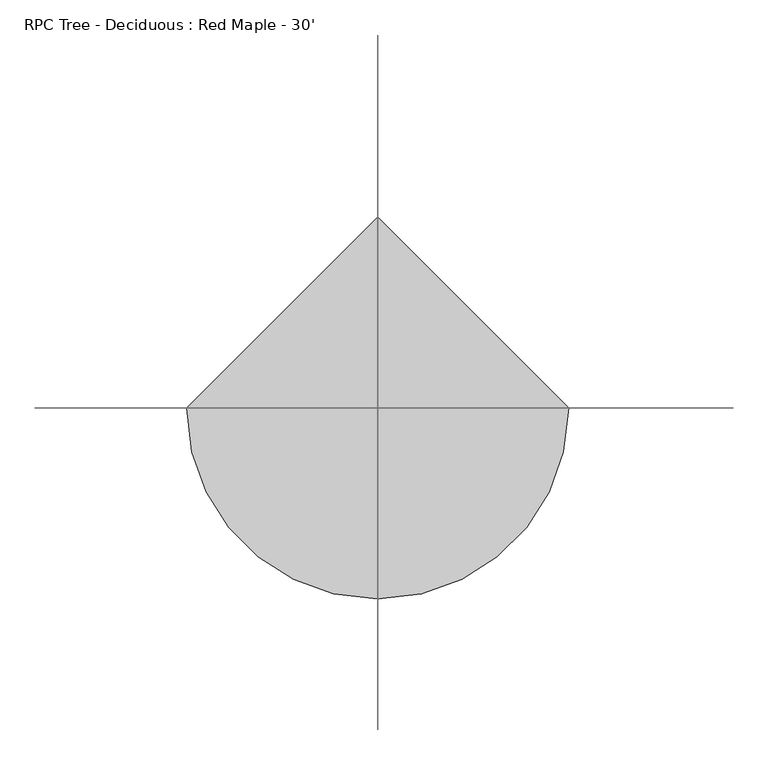
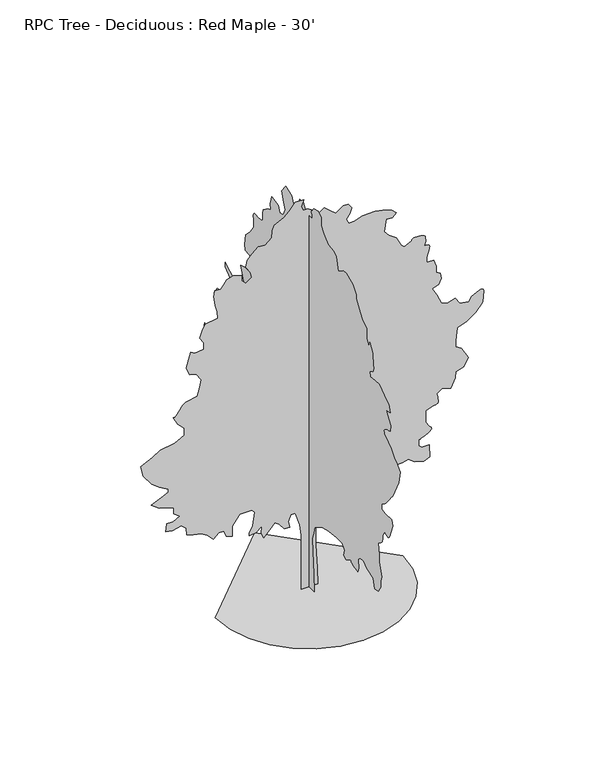
"""IFC4 building model written with IfcOpenShell, lengths in millimetres: geographic element geometry, RPC Tree - Deciduous : Red Maple - 30'."""

from ifc_helpers import new_model, si_unit, origin, place, context, project, spatial, triangles, source, transform, mapped, element, save


def rpc_tree_deciduous_red_maple_30_cba750cc(model_context):
    return source(origin(), model_context, "Body", "Tessellation", [
        triangles([(5.9e-06, 200.5240248, 0.0131599), (5.9e-06, -200.5423013, 0.0131599), (5.9e-06, -173.8047255, 401.079007), (5.9e-06, -147.0663684, 922.4677488), (5.9e-06, -133.6980892, 1216.5822092), (5.9e-06, -173.8047255, 1363.6407475), (5.9e-06, -227.2806583, 1537.4352264), (5.9e-06, -320.8632274, 1590.9124855), (5.9e-06, -534.7644153, 1711.2323215), (5.9e-06, -762.0361897, 1764.7071098), (5.9e-06, -1069.5212002, 1804.8136734), (5.9e-06, -1283.4223881, 1804.8136734), (5.9e-06, -1377.0037399, 1697.8617714), (5.9e-06, -1336.897031, 1550.8033058), (5.9e-06, -1443.848933, 1510.6967422), (5.9e-06, -1617.6460281, 1604.2805649), (5.9e-06, -1620.762553, 1592.8200726), (5.9e-06, -1625.400642, 1581.362051), (5.9e-06, -1633.0790977, 1569.9041748), (5.9e-06, -1645.319339, 1558.4436825), (5.9e-06, -1663.6378429, 1546.9856609), (5.9e-06, -1689.5560284, 1535.5251686), (5.9e-06, -1724.595314, 1524.0672924), (5.9e-06, -1761.1942429, 1514.1662979), (5.9e-06, -1791.4812023, 1507.0721088), (5.9e-06, -1816.5027855, 1502.3197826), (5.9e-06, -1837.3156139, 1499.4343483), (5.9e-06, -1854.971077, 1497.9534794), (5.9e-06, -1870.5234707, 1497.4074371), (5.9e-06, -1885.021859, 1497.3286629), (5.9e-06, -1911.7604885, 1590.9124855), (5.9e-06, -1898.3924091, 1791.445594), (5.9e-06, -1978.6056816, 1871.6588665), (5.9e-06, -2112.293597, 1885.0269459), (5.9e-06, -2219.245499, 1778.0750439), (5.9e-06, -2473.2533958, 1697.8617714), (5.9e-06, -2540.1036758, 1497.3286629), (5.9e-06, -2660.4236572, 1510.6967422), (5.9e-06, -2767.3575371, 1671.125758), (5.9e-06, -2767.3575371, 1804.8136734), (5.9e-06, -2794.1038696, 1911.7655754), (5.9e-06, -2700.5302208, 2219.2479698), (5.9e-06, -2700.5302208, 2393.0450649), (5.9e-06, -2673.7838882, 2660.4236572), (5.9e-06, -2676.8572472, 2660.5759735), (5.9e-06, -2681.2261665, 2661.668058), (5.9e-06, -2688.1603363, 2664.6399696), (5.9e-06, -2698.9553169, 2670.4056061), (5.9e-06, -2714.9066689, 2679.9053169), (5.9e-06, -2737.284082, 2694.1038689), (5.9e-06, -2767.3575371, 2713.8904518), (5.9e-06, -2796.66912, 2738.3761665), (5.9e-06, -2816.8623642, 2765.6558968), (5.9e-06, -2829.4607231, 2795.2721123), (5.9e-06, -2835.9629425, 2826.7681549), (5.9e-06, -2837.9189278, 2859.6612053), (5.9e-06, -2836.8265526, 2893.4940239), (5.9e-06, -2834.2104332, 2927.8096619), (5.9e-06, -2914.423851, 3061.4898743), (5.9e-06, -2945.8434448, 3041.8556076), (5.9e-06, -2976.6790627, 3024.6598549), (5.9e-06, -3006.3211487, 3012.3917084), (5.9e-06, -3034.2357239, 3007.4641022), (5.9e-06, -3059.8135231, 3012.3917084), (5.9e-06, -3082.4449905, 3029.5618813), (5.9e-06, -3101.5964378, 3061.4898743), (5.9e-06, -3235.2766502, 3382.3429642), (5.9e-06, -3195.1700867, 3516.0231766), (5.9e-06, -2941.1698929, 3502.6629456), (5.9e-06, -2794.1038696, 3516.0231766), (5.9e-06, -2807.4641006, 3649.7289688), (5.9e-06, -2841.8811859, 3670.0236603), (5.9e-06, -2876.5523254, 3691.8420959), (5.9e-06, -2911.6551247, 3716.7088921), (5.9e-06, -2947.4692177, 3746.1475021), (5.9e-06, -2984.2230789, 3781.6566719), (5.9e-06, -3022.1707626, 3824.7604362), (5.9e-06, -3061.4898743, 3876.98283), (5.9e-06, -3098.0914192, 3928.4433517), (5.9e-06, -3128.3680595, 3969.3626564), (5.9e-06, -3153.3871719, 4001.5191238), (5.9e-06, -3174.2152611, 4026.6652634), (5.9e-06, -3191.8682533, 4046.5280045), (5.9e-06, -3207.412944, 4062.9110161), (5.9e-06, -3221.9164192, 4077.5159386), (5.9e-06, -3449.1958603, 4532.0748207), (5.9e-06, -3516.0231766, 4826.1815781), (5.9e-06, -3368.9824425, 4986.6084137), (5.9e-06, -3302.1295464, 4999.9686447), (5.9e-06, -3155.0635231, 5187.1415222), (5.9e-06, -3061.4898743, 5253.9944183), (5.9e-06, -3024.5075386, 5271.2916183), (5.9e-06, -2989.023658, 5289.3004028), (5.9e-06, -2956.5878471, 5308.7056137), (5.9e-06, -2928.7238503, 5330.2194168), (5.9e-06, -2906.9559929, 5354.5528152), (5.9e-06, -2892.7574409, 5382.3656525), (5.9e-06, -2887.6775185, 5414.4206726), (5.9e-06, -2894.7134262, 5445.6629517), (5.9e-06, -2914.3474022, 5471.3166183), (5.9e-06, -2944.5228859, 5492.2973145), (5.9e-06, -2983.1054146, 5509.5183563), (5.9e-06, -3028.0125572, 5523.9453827), (5.9e-06, -3077.1107231, 5536.493454), (5.9e-06, -3128.3171906, 5548.100885), (5.9e-06, -3141.7030014, 5695.1669083), (5.9e-06, -3074.850396, 5802.1010788), (5.9e-06, -2967.8906456, 5949.1671021), (5.9e-06, -3128.3171906, 5989.2739563), (5.9e-06, -3074.850396, 6149.7007919), (5.9e-06, -2901.0633293, 6256.6599609), (5.9e-06, -2700.5302208, 6403.7009857), (5.9e-06, -2526.7306549, 6390.3401733), (5.9e-06, -2366.3039646, 6376.9799423), (5.9e-06, -2339.5653351, 6483.9141129), (5.9e-06, -2419.7786076, 6537.4061966), (5.9e-06, -2434.0052101, 6540.4798462), (5.9e-06, -2447.6476913, 6544.8487656), (5.9e-06, -2460.1190231, 6551.7826447), (5.9e-06, -2470.8378456, 6562.577916), (5.9e-06, -2479.217276, 6578.5292679), (5.9e-06, -2484.6730476, 6600.9063904), (5.9e-06, -2486.6238007, 6630.9801361), (5.9e-06, -2485.4529419, 6668.4702896), (5.9e-06, -2482.1813393, 6711.5746353), (5.9e-06, -2477.1522858, 6759.3769501), (5.9e-06, -2470.7209923, 6810.8883408), (5.9e-06, -2463.2380188, 6865.2193268), (5.9e-06, -2455.0515999, 6921.4292679), (5.9e-06, -2446.5172371, 6978.5792679), (5.9e-06, -2339.5653351, 7165.7521454), (5.9e-06, -2299.4587715, 7058.792395), (5.9e-06, -2232.6135784, 7179.1123764), (5.9e-06, -2232.6135784, 7433.1125702), (5.9e-06, -2058.8189541, 7540.0723206), (5.9e-06, -1938.499118, 7700.4985748), (5.9e-06, -1818.1791367, 7874.2856415), (5.9e-06, -1818.1791367, 7967.8845795), (5.9e-06, -1684.4887505, 8128.3114151), (5.9e-06, -1443.848933, 8248.6313965), (5.9e-06, -1310.1610176, 8221.8847733), (5.9e-06, -1136.3639225, 8101.5647919), (5.9e-06, -1042.7825706, 8395.6718399), (5.9e-06, -949.198748, 8462.524736), (5.9e-06, -735.2975601, 8489.2707779), (5.9e-06, -574.8710515, 8649.6976135), (5.9e-06, -467.9217293, 8770.0175949), (5.9e-06, -467.9217293, 8957.1648926), (5.9e-06, -347.6018206, 9037.3780197), (5.9e-06, -187.1730047, 8997.2711655), (5.9e-06, -93.5917073, 8876.9517654), (5.9e-06, -107.5840764, 8845.6589081), (5.9e-06, -119.5886307, 8815.6357407), (5.9e-06, -127.6175737, 8788.2036942), (5.9e-06, -129.6833633, 8764.6324585), (5.9e-06, -123.7979213, 8746.192305), (5.9e-06, -107.9734512, 8734.1779221), (5.9e-06, -80.2224107, 8729.9107407), (5.9e-06, 106.9427183, 8729.9107407), (5.9e-06, 227.262618, 8903.6978073), (5.9e-06, 360.9520595, 8890.3375763), (5.9e-06, 427.7947454, 8729.9107407), (5.9e-06, 601.5918769, 8649.6976135), (5.9e-06, 668.4345629, 8783.3778259), (5.9e-06, 895.7063009, 8876.9517654), (5.9e-06, 1042.7648392, 8676.4180756), (5.9e-06, 975.9195734, 8449.164505), (5.9e-06, 922.4449305, 8302.0984818), (5.9e-06, 989.2901236, 8141.6716461), (5.9e-06, 1122.9781116, 8114.9256042), (5.9e-06, 1176.4527546, 8261.9916275), (5.9e-06, 1443.8312016, 8288.7376694), (5.9e-06, 1497.3083153, 8101.5647919), (5.9e-06, 1470.5696857, 7967.8845795), (5.9e-06, 1590.8896671, 7927.7783066), (5.9e-06, 1764.6841461, 7794.0725143), (5.9e-06, 1778.0546963, 7700.4985748), (5.9e-06, 1778.0546963, 7540.0723206), (5.9e-06, 1844.8974186, 7499.9654663), (5.9e-06, 2005.3239635, 7499.9654663), (5.9e-06, 2036.5838287, 7505.2994431), (5.9e-06, 2066.3221298, 7508.2969345), (5.9e-06, 2093.0200642, 7506.6202927), (5.9e-06, 2115.1586838, 7497.9336136), (5.9e-06, 2131.2167152, 7479.8998306), (5.9e-06, 2139.6749199, 7450.1562973), (5.9e-06, 2139.0144951, 7406.3921082), (5.9e-06, 2134.0639252, 7358.3095779), (5.9e-06, 2130.5182114, 7316.5772415), (5.9e-06, 2128.1407402, 7280.1033051), (5.9e-06, 2126.6979504, 7247.8198105), (5.9e-06, 2125.9562805, 7218.7111221), (5.9e-06, 2125.6844948, 7191.6854462), (5.9e-06, 2125.6464157, 7165.7521454), (5.9e-06, 2259.3343311, 6978.5792679), (5.9e-06, 2433.1289555, 6804.7922012), (5.9e-06, 2473.2356644, 6550.767009), (5.9e-06, 2446.4995056, 6430.4470276), (5.9e-06, 2312.8089741, 6417.0867966), (5.9e-06, 2205.8596882, 6390.3401733), (5.9e-06, 2125.6464157, 6216.5531067), (5.9e-06, 2232.5957016, 6016.0199982), (5.9e-06, 2473.2356644, 6016.0199982), (5.9e-06, 2633.6520355, 5962.5279144), (5.9e-06, 2499.9741486, 5614.9537811), (5.9e-06, 2620.2915138, 5481.2479889), (5.9e-06, 2954.5048347, 5521.3548431), (5.9e-06, 3048.1040634, 5574.8475082), (5.9e-06, 3235.2513611, 5668.4208664), (5.9e-06, 3221.8908394, 5574.8475082), (5.9e-06, 2981.2511673, 5360.9280075), (5.9e-06, 2887.6775185, 5066.8215408), (5.9e-06, 2994.611689, 4839.5420998), (5.9e-06, 3141.6777122, 4852.9279106), (5.9e-06, 3144.9033875, 4867.1011734), (5.9e-06, 3150.3643913, 4880.4869843), (5.9e-06, 3160.2704727, 4892.2217331), (5.9e-06, 3176.8313805, 4901.4926788), (5.9e-06, 3202.2821526, 4907.4870804), (5.9e-06, 3238.8581177, 4909.3921967), (5.9e-06, 3288.7437355, 4906.3947052), (5.9e-06, 3529.3836983, 4879.6486633), (5.9e-06, 3649.703389, 4705.8618874), (5.9e-06, 3609.5968254, 4518.6890099), (5.9e-06, 3462.5308022, 4411.7548393), (5.9e-06, 3342.2108208, 4117.6227928), (5.9e-06, 3395.677906, 3930.4752045), (5.9e-06, 3449.1702805, 3863.622599), (5.9e-06, 3582.8507835, 3636.343158), (5.9e-06, 3850.2367882, 3663.0891998), (5.9e-06, 4024.0235641, 3770.0489502), (5.9e-06, 4077.4906494, 3529.4089874), (5.9e-06, 3823.4904556, 3409.089006), (5.9e-06, 3649.703389, 3355.5966316), (5.9e-06, 3529.3836983, 3088.2362068), (5.9e-06, 3462.5308022, 2927.8096619), (5.9e-06, 3382.3173843, 2700.5302208), (5.9e-06, 3235.2513611, 2727.2762627), (5.9e-06, 3007.9974998, 2767.3831169), (5.9e-06, 2820.8246223, 2727.2762627), (5.9e-06, 2687.1444099, 2513.364901), (5.9e-06, 2860.9311859, 2339.570422), (5.9e-06, 3021.3577309, 2312.8319378), (5.9e-06, 3048.1040634, 2058.8215702), (5.9e-06, 3036.4454727, 2033.2918785), (5.9e-06, 3023.6183487, 2009.2838963), (5.9e-06, 3008.4547394, 1988.3135193), (5.9e-06, 2989.7855301, 1971.9052185), (5.9e-06, 2966.4430595, 1961.5775059), (5.9e-06, 2937.258213, 1958.8496201), (5.9e-06, 2901.0380402, 1965.2402184), (5.9e-06, 2863.2679619, 1977.8690987), (5.9e-06, 2829.7147774, 1992.6010483), (5.9e-06, 2799.6663208, 2009.0882687), (5.9e-06, 2772.4121704, 2026.9800545), (5.9e-06, 2747.2916107, 2045.9209042), (5.9e-06, 2723.5424789, 2065.5651993), (5.9e-06, 2700.504641, 2085.5600544), (5.9e-06, 2606.9309921, 2192.5119564), (5.9e-06, 2589.5829231, 2220.7695339), (5.9e-06, 2571.2947952, 2246.6877193), (5.9e-06, 2551.1527107, 2267.9297367), (5.9e-06, 2528.193647, 2282.1561939), (5.9e-06, 2501.4929512, 2287.0279896), (5.9e-06, 2470.1189941, 2280.208057), (5.9e-06, 2433.1289555, 2259.3571495), (5.9e-06, 2386.7865807, 2232.2681053), (5.9e-06, 2329.2174202, 2207.9857212), (5.9e-06, 2262.2959236, 2186.0425838), (5.9e-06, 2187.8891281, 2165.9689545), (5.9e-06, 2107.8714832, 2147.2998905), (5.9e-06, 2024.1123516, 2129.5656532), (5.9e-06, 1938.4812412, 2112.2986839), (5.9e-06, 1724.5775826, 2058.8215702), (5.9e-06, 1791.4227757, 1925.1335094), (5.9e-06, 2005.3239635, 1791.445594), (5.9e-06, 2112.2758656, 1617.6484989), (5.9e-06, 1925.1106911, 1550.8033058), (5.9e-06, 1899.2305847, 1550.9989334), (5.9e-06, 1872.766357, 1552.362949), (5.9e-06, 1845.1311253, 1556.0662113), (5.9e-06, 1815.7433842, 1563.2772537), (5.9e-06, 1784.0161057, 1575.1644642), (5.9e-06, 1749.3654591, 1592.8988468), (5.9e-06, 1711.2095032, 1617.6484989), (5.9e-06, 1671.8826885, 1646.6858253), (5.9e-06, 1633.9579685, 1676.4242718), (5.9e-06, 1597.2041073, 1706.7493103), (5.9e-06, 1561.3849274, 1737.539146), (5.9e-06, 1526.2668674, 1768.6821579), (5.9e-06, 1491.6162209, 1800.0587311), (5.9e-06, 1457.1991356, 1831.5523029), (5.9e-06, 1189.8233047, 1911.7655754), (5.9e-06, 975.9195734, 1951.872139), (5.9e-06, 762.0183855, 2005.3467819), (5.9e-06, 548.1146542, 1965.2402184), (5.9e-06, 253.9999576, 1858.2883163), (5.9e-06, 173.7866851, 1751.3390305), (5.9e-06, 106.9427183, 1564.173856), (5.9e-06, 80.2041161, 1296.7955544), (5.9e-06, 106.9427183, 935.8358282), (5.9e-06, 160.4173885, 414.4495934), (-2085.2019367, 0.0, 0.0), (-2030.0762318, -477.7896226, 0.0), (-1873.078838, -916.5648388, 0.0), (-1626.7799183, -1303.7500717, 0.0), (-1303.7500717, -1626.7799183, 0.0), (-916.5648388, -1873.078838, 0.0), (-477.7896226, -2030.0762318, 0.0), (9.11e-05, -2085.2019367, 0.0), (477.7896226, -2030.0762318, 0.0), (916.5648388, -1873.078838, 0.0), (1303.7500717, -1626.7799183, 0.0), (1626.7799183, -1303.7500717, 0.0), (1873.078838, -916.5648388, 0.0), (2030.0762318, -477.7896226, 0.0), (2085.2019367, 0.0001828, 0.0), (-0.0002734, 2085.2019367, 0.0), (199.8874902, 0.0002285, 0.005264), (-169.704903, 0.0002285, 0.005264), (-169.704903, 0.0001919, 684.4365658), (-169.704903, 0.0001645, 1040.3416586), (-169.704903, 0.0001554, 1273.0464226), (-210.770892, 0.0001371, 1533.1325821), (-306.5909517, 0.0001188, 1834.2801888), (-402.4125375, 0.0001188, 1834.2801888), (-457.1673348, 0.0001279, 1683.7063854), (-429.7886644, 0.0001371, 1546.8205547), (-552.9863771, 0.0001371, 1560.5086727), (-662.4960445, 0.0001279, 1697.3945034), (-758.317594, 0.0001279, 1765.8374187), (-867.8247179, 0.0001279, 1642.639706), (-1004.7104759, 0.0001371, 1505.7538754), (-1059.465346, 0.0001371, 1628.9515881), (-1045.777228, 0.0001279, 1793.2159801), (-1182.6630587, 0.0001279, 1683.7063854), (-1333.2394054, 0.0001279, 1670.0182674), (-1333.2394054, 0.0001279, 1738.4611828), (-1251.1059013, 0.0001188, 1875.3470135), (-1210.0416927, 0.0001005, 2176.4972363), (-1278.4846081, 0.0001005, 2244.9401516), (-1538.5681515, 0.0001005, 2244.9401516), (-1702.8300728, 0.0001097, 2012.2328442), (-1702.8300728, 0.0001188, 1916.4136929), (-1702.8300728, 0.0001279, 1779.5280075), (-1839.7183743, 0.0001188, 1834.2801888), (-1894.4731716, 0.0001097, 1971.1686356), (-2003.9802956, 0.0001097, 1971.1686356), (-2127.1780083, 0.0001188, 1861.6588955), (-2264.063839, 0.0001097, 1998.5447262), (-2400.9521404, 0.0001097, 2080.6756142), (-2578.9149696, 0.0001005, 2121.7424389), (-2715.7955681, 0.0001005, 2176.4972363), (-2729.4863022, 9.14e-05, 2327.0711849), (-2838.9857231, 8.22e-05, 2422.8926617), (-3044.3194107, 9.14e-05, 2381.8259823), (-3181.2000092, 8.22e-05, 2409.204689), (-3167.5095657, 7.31e-05, 2587.1444092), (-3016.9382332, 7.31e-05, 2587.1444092), (-2880.0576347, 7.31e-05, 2669.2882324), (-3003.2474991, 6.4e-05, 2765.0969193), (-3003.2474991, 5.48e-05, 2902.0030975), (-3140.1283882, 5.48e-05, 2956.7401634), (-3331.7713417, 5.48e-05, 3011.5025185), (-3509.7241425, 4.57e-05, 3148.3834076), (-3290.6997208, 3.66e-05, 3244.2176743), (-3126.4376541, 3.66e-05, 3312.6451836), (-3126.4376541, 2.74e-05, 3381.0982727), (-3331.7713417, 1.83e-05, 3504.2884277), (-3496.0334084, 1.83e-05, 3627.5038719), (-3687.6766525, 0.0, 3887.5746254), (-3742.4390076, -1.83e-05, 4133.9802246), (-3632.9395866, -1.83e-05, 4188.7172905), (-3482.3426743, -2.74e-05, 4257.1703796), (-3304.3901642, -2.74e-05, 4366.6698006), (-2989.5570557, -3.66e-05, 4421.4324463), (-2770.532634, -3.66e-05, 4530.9318672), (-2770.532634, -4.57e-05, 4695.1936432), (-2921.1292557, -5.48e-05, 4845.7905556), (-3016.9382332, -7.31e-05, 5023.742775), (-3007.9974998, -7.31e-05, 5021.1266556), (-2998.2184456, -7.31e-05, 5020.5679688), (-2986.7630402, -7.31e-05, 5024.0985672), (-2972.7929626, -7.31e-05, 5033.6997253), (-2955.4701828, -7.31e-05, 5051.4544556), (-2933.9816689, -7.31e-05, 5079.3946106), (-2907.4388123, -7.31e-05, 5119.5520432), (-2879.295472, -7.31e-05, 5162.0971207), (-2853.3113022, -8.22e-05, 5196.7426804), (-2829.1305107, -8.22e-05, 5224.783992), (-2806.3720161, -8.22e-05, 5247.5680664), (-2784.7058968, -8.22e-05, 5266.4145905), (-2763.7507805, -8.22e-05, 5282.6199966), (-2743.1767456, -8.22e-05, 5297.5045532), (-2483.0830284, -9.14e-05, 5352.2669083), (-2428.328231, -0.0001005, 5543.9098618), (-2400.9521404, -0.0001097, 5708.1719284), (-2510.4618805, -0.0001188, 5872.4339951), (-2647.3424789, -0.0001188, 5913.4803268), (-2729.4863022, -0.0001371, 6091.4328369), (-2674.7236565, -0.0001462, 6283.0757904), (-2633.6520355, -0.0001554, 6433.6474136), (-2537.8378258, -0.0001462, 6378.9100571), (-2346.1973431, -0.0001554, 6406.2915253), (-2346.1973431, -0.0001645, 6556.8625671), (-2428.328231, -0.0001645, 6693.7437469), (-2373.5734337, -0.0001736, 6844.3147888), (-2305.1305183, -0.0001828, 6981.1953873), (-2031.3590023, -0.0001919, 7022.2672989), (-2045.0471203, -0.0002011, 7186.5293655), (-2086.1137997, -0.0002102, 7337.1004074), (-2113.4900356, -0.0002193, 7556.1248291), (-2099.8019176, -0.0002285, 7693.0060089), (-1962.916087, -0.0002285, 7679.3149841), (-1894.4731716, -0.0002285, 7761.4588074), (-1826.0302563, -0.0002376, 7857.2674942), (-1689.1419548, -0.0002376, 7898.3394058), (-1497.5013268, -0.0002376, 7843.5770508), (-1497.5013268, -0.0002285, 7720.3868958), (-1401.6823208, -0.0002285, 7624.5782089), (-1278.4846081, -0.0002285, 7720.3868958), (-1305.8606987, -0.0002376, 7857.2674942), (-1401.6823208, -0.0002467, 8007.8391174), (-1374.303614, -0.0002559, 8158.4357391), (-1264.7940193, -0.000265, 8267.9354507), (-1127.9081886, -0.0002742, 8391.1250244), (-977.3343853, -0.000265, 8377.434581), (-826.7605093, -0.0002742, 8500.6503159), (-813.0699205, -0.0002833, 8651.2213577), (-772.0057119, -0.0002924, 8774.4115128), (-566.6744588, -0.0003016, 8870.2457794), (-443.4767461, -0.0003016, 8979.745491), (-306.5909517, -0.0003107, 9144.0075577), (-114.9505871, -0.0003107, 9144.0075577), (-169.704903, -0.0003016, 8993.4359344), (-128.6391684, -0.0003016, 8897.6016678), (-32.8188589, -0.0003016, 8897.6016678), (49.3128694, -0.0002924, 8842.8648926), (76.6900319, -0.0002924, 8733.3396011), (240.9532249, -0.0002924, 8719.6491577), (336.7737751, -0.0002924, 8788.1019562), (473.6595695, -0.0002833, 8678.6028259), (596.8572822, -0.0002833, 8569.0781158), (761.1217833, -0.0002833, 8692.2932693), (870.6314507, -0.0002833, 8692.2932693), (952.7624113, -0.0002833, 8582.7685593), (911.6956593, -0.0002742, 8445.8879608), (829.5646986, -0.000265, 8350.0786926), (884.319496, -0.000265, 8240.5539825), (1007.5172087, -0.000265, 8240.5539825), (1199.1578367, -0.000265, 8309.006781), (1472.9294254, -0.000265, 8309.006781), (1637.1938175, -0.000265, 8281.6258942), (1842.5225636, -0.0002559, 8213.1725143), (1938.3441856, -0.0002559, 8117.3638275), (1856.2106815, -0.0002467, 8021.5295609), (1719.3248508, -0.0002467, 8035.2200043), (1691.9487602, -0.0002376, 7912.0298492), (1678.2580261, -0.0002285, 7761.4588074), (1774.0796482, -0.0002285, 7638.2686523), (1938.3441856, -0.0002193, 7528.7439423), (2047.8513096, -0.0002011, 7309.7195206), (2116.2940796, -0.0002011, 7254.982164), (2280.558617, -0.0002102, 7337.1004074), (2283.7919952, -0.0002102, 7348.7589981), (2288.8187233, -0.0002102, 7359.9350601), (2297.439418, -0.0002102, 7370.1460648), (2311.4475746, -0.0002102, 7378.9344818), (2332.6388683, -0.0002102, 7385.7927841), (2362.8089745, -0.0002102, 7390.2628601), (2403.7563297, -0.0002102, 7391.8633438), (2446.2989365, -0.0002102, 7390.2628601), (2480.9392639, -0.0002102, 7385.7927841), (2508.9962723, -0.0002102, 7378.9344818), (2531.7826721, -0.0002102, 7370.1460648), (2550.619313, -0.0002102, 7359.9350601), (2566.8244286, -0.0002102, 7348.7589981), (2581.7089851, -0.0002102, 7337.1004074), (2595.3994286, -0.0002011, 7213.9108337), (2568.018251, -0.0001919, 7118.1015656), (2599.8953751, -0.0001919, 7117.6446167), (2629.5115906, -0.0001919, 7114.5709671), (2654.581572, -0.0001919, 7106.2400803), (2672.8188309, -0.0001919, 7089.9840958), (2681.9627495, -0.0001919, 7063.2124741), (2679.7274208, -0.0001919, 7023.2579361), (2663.8525177, -0.0001828, 6967.5049438), (2643.9641968, -0.0001828, 6908.5771454), (2630.5530968, -0.0001828, 6859.6818741), (2622.5268425, -0.0001736, 6819.1686493), (2618.8183479, -0.0001736, 6785.3614105), (2618.3358192, -0.0001736, 6756.6085144), (2620.0121704, -0.0001736, 6731.1833221), (2622.7806061, -0.0001736, 6707.4341904), (2773.3519386, -0.0001736, 6707.4341904), (2828.1145844, -0.0001554, 6543.1721237), (2828.1145844, -0.0001554, 6406.2915253), (2923.9232712, -0.0001462, 6351.5291702), (2937.6140053, -0.0001371, 6228.3390152), (2882.8516502, -0.0001371, 6105.1232803), (2745.9707611, -0.0001279, 6050.3865051), (2841.8050278, -0.0001188, 5872.4339951), (2937.6140053, -0.0001097, 5653.4095734), (3074.4946037, -0.0001005, 5584.9561935), (3252.4471138, -0.0001097, 5639.7191299), (3348.2813805, -0.0001005, 5489.1475067), (3553.5897789, -9.14e-05, 5461.7666199), (3622.042868, -0.0001005, 5557.5753067), (3677.3894897, -0.0001005, 5589.3251129), (3730.4754936, -0.0001005, 5617.7989563), (3779.0149727, -0.0001097, 5639.8458664), (3820.6964401, -0.0001097, 5652.1648819), (3853.3101471, -0.0001097, 5651.5806152), (3874.5446068, -0.0001097, 5634.8165222), (3882.1392014, -0.0001005, 5598.6472183), (3881.3261696, -0.0001005, 5553.3081253), (3879.0911316, -0.0001005, 5510.8647858), (3875.6619804, -9.14e-05, 5470.7835114), (3871.2677719, -9.14e-05, 5432.6323517), (3866.1625603, -9.14e-05, 5395.9293594), (3860.5745293, -9.14e-05, 5360.1664261), (3854.7580238, -9.14e-05, 5324.8854401), (3704.1866913, -7.31e-05, 5160.6239548), (3512.5434471, -6.4e-05, 5010.0523315), (3293.5190254, -6.4e-05, 4941.5995331), (3266.1378479, -4.57e-05, 4640.4565773), (3266.1378479, -3.66e-05, 4503.5506897), (3389.3280029, -3.66e-05, 4421.4324463), (3539.9246246, -1.83e-05, 4161.336113), (3444.090358, -9.1e-06, 3969.7184486), (3266.1378479, 0.0, 3914.9558029), (3252.4471138, 9.1e-06, 3778.0752045), (3156.638427, 1.83e-05, 3559.0507828), (2964.9951828, 1.83e-05, 3627.5038719), (2846.3771324, 1.83e-05, 3536.8765549), (2845.4879425, 1.83e-05, 3538.3244316), (2845.1071518, 1.83e-05, 3537.5369797), (2845.7675766, 1.83e-05, 3532.3047409), (2847.9773254, 1.83e-05, 3520.3665161), (2852.269796, 1.83e-05, 3499.5131378), (2859.1786766, 2.74e-05, 3467.5345665), (2869.1609161, 2.74e-05, 3422.1701843), (2875.307634, 2.74e-05, 3376.1453773), (2871.3959541, 2.74e-05, 3342.3378479), (2859.1025185, 3.66e-05, 3318.7157433), (2840.1286766, 3.66e-05, 3303.2219215), (2816.1002014, 3.66e-05, 3293.8492378), (2788.7190239, 3.66e-05, 3288.5405502), (2759.6614952, 3.66e-05, 3285.264006), (2595.3994286, 3.66e-05, 3230.5269402), (2595.3994286, 5.48e-05, 2956.7401634), (2677.517672, 6.4e-05, 2833.5500084), (2697.53302, 6.4e-05, 2815.871727), (2714.297113, 6.4e-05, 2797.7106262), (2724.5839851, 6.4e-05, 2778.5844681), (2725.1682518, 6.4e-05, 2758.0357224), (2712.8492363, 6.4e-05, 2735.582151), (2684.3503944, 7.31e-05, 2710.7156456), (2636.4713402, 7.31e-05, 2682.9786758), (2584.1727882, 7.31e-05, 2657.2229805), (2543.4055092, 7.31e-05, 2637.9697952), (2512.1864845, 7.31e-05, 2624.0761665), (2488.640538, 7.31e-05, 2614.5002975), (2470.8427872, 7.31e-05, 2608.1503944), (2456.8753258, 7.31e-05, 2603.9593712), (2444.8231544, 7.31e-05, 2600.8351433), (2444.8231544, 8.22e-05, 2463.9594864), (2513.2660698, 9.14e-05, 2395.5139549), (2677.517672, 9.14e-05, 2395.5139549), (2691.2084061, 0.0001005, 2108.0543209), (2554.3275169, 0.0001097, 2053.2995235), (2349.0015324, 0.0001005, 2121.7424389), (2212.1157017, 0.0001005, 2217.564061), (2075.229871, 0.0001005, 2190.1853542), (1828.8344456, 0.0001005, 2176.4972363), (1678.2580261, 0.0001005, 2135.4305569), (1664.5700535, 0.0001188, 1943.7899288), (1513.9961048, 0.0001188, 1930.1018108), (1322.3554768, 0.0001188, 1943.7899288), (1240.2219727, 0.0001188, 1820.5922161), (952.7624113, 0.0001279, 1779.5280075), (733.7430765, 0.0001188, 1834.2801888), (733.7430765, 0.0001371, 1615.2634701), (555.7930736, 0.0001371, 1628.9515881), (501.0382762, 0.0001279, 1738.4611828), (405.2166904, 0.0001279, 1697.3945034), (295.7070412, 0.0001279, 1697.3945034), (254.6428326, 0.0001188, 1820.5922161), (145.13292, 0.0001279, 1697.3945034), (131.4443387, 0.0001371, 1546.8205547), (145.13292, 0.0001554, 1314.1132473), (145.13292, 0.0001736, 930.8319912), (186.1989181, 0.0002102, 383.2863067)], [[130, 131, 132], [208, 209, 210], [208, 210, 211], [207, 208, 211], [230, 231, 232], [230, 232, 233], [276, 277, 278], [229, 230, 233], [229, 233, 234], [302, 1, 2], [302, 2, 3], [302, 3, 4], [301, 302, 4], [301, 4, 5], [300, 301, 5], [300, 5, 6], [299, 300, 6], [299, 6, 7], [108, 109, 110], [203, 204, 205], [206, 207, 211], [206, 211, 212], [108, 110, 111], [202, 203, 205], [13, 14, 15], [13, 15, 16], [236, 237, 238], [171, 172, 173], [170, 171, 173], [170, 173, 174], [36, 37, 38], [36, 38, 39], [36, 39, 40], [275, 276, 278], [275, 278, 279], [275, 279, 280], [275, 280, 281], [275, 281, 282], [275, 282, 283], [275, 283, 284], [275, 284, 285], [275, 285, 286], [275, 286, 287], [275, 287, 288], [275, 288, 289], [275, 289, 290], [274, 275, 290], [274, 290, 291], [274, 291, 292], [67, 68, 69], [66, 67, 69], [164, 165, 166], [164, 166, 167], [163, 164, 167], [163, 167, 168], [242, 243, 244], [29, 30, 31], [104, 105, 106], [197, 198, 199], [28, 29, 31], [298, 299, 7], [66, 69, 70], [65, 66, 70], [64, 65, 70], [63, 64, 70], [62, 63, 70], [61, 62, 70], [60, 61, 70], [59, 60, 70], [27, 28, 31], [150, 151, 152], [160, 161, 162], [159, 160, 162], [196, 197, 199], [195, 196, 199], [195, 199, 200], [26, 27, 31], [133, 134, 135], [242, 244, 245], [242, 245, 246], [242, 246, 247], [242, 247, 248], [242, 248, 249], [242, 249, 250], [242, 250, 251], [242, 251, 252], [242, 252, 253], [242, 253, 254], [242, 254, 255], [242, 255, 256], [242, 256, 257], [242, 257, 258], [242, 258, 259], [241, 242, 259], [241, 259, 260], [241, 260, 261], [241, 261, 262], [241, 262, 263], [241, 263, 264], [298, 7, 8], [274, 292, 293], [147, 148, 149], [147, 149, 150], [147, 150, 152], [147, 152, 153], [147, 153, 154], [147, 154, 155], [147, 155, 156], [36, 40, 41], [36, 41, 42], [35, 36, 42], [34, 35, 42], [34, 42, 43], [86, 87, 88], [86, 88, 89], [34, 43, 44], [104, 106, 107], [103, 104, 107], [102, 103, 107], [25, 26, 31], [25, 31, 32], [24, 25, 32], [23, 24, 32], [22, 23, 32], [21, 22, 32], [20, 21, 32], [19, 20, 32], [18, 19, 32], [17, 18, 32], [16, 17, 32], [13, 16, 32], [12, 13, 32], [102, 107, 108], [101, 102, 108], [129, 130, 132], [146, 147, 156], [100, 101, 108], [236, 238, 239], [146, 156, 157], [221, 222, 223], [221, 223, 224], [221, 224, 225], [220, 221, 225], [219, 220, 225], [218, 219, 225], [217, 218, 225], [216, 217, 225], [215, 216, 225], [214, 215, 225], [213, 214, 225], [213, 225, 226], [33, 34, 44], [235, 236, 239], [298, 8, 9], [297, 298, 9], [12, 32, 33], [58, 59, 70], [175, 176, 177], [85, 86, 89], [85, 89, 90], [85, 90, 91], [85, 91, 92], [84, 85, 92], [84, 92, 93], [83, 84, 93], [82, 83, 93], [82, 93, 94], [81, 82, 94], [80, 81, 94], [80, 94, 95], [79, 80, 95], [12, 33, 44], [78, 79, 95], [77, 78, 95], [76, 77, 95], [75, 76, 95], [74, 75, 95], [73, 74, 95], [72, 73, 95], [71, 72, 95], [71, 95, 96], [108, 111, 112], [108, 112, 113], [100, 108, 113], [100, 113, 114], [99, 100, 114], [98, 99, 114], [194, 195, 200], [128, 129, 132], [137, 138, 139], [175, 177, 178], [174, 175, 178], [241, 264, 265], [139, 140, 141], [139, 141, 142], [137, 139, 142], [229, 234, 235], [229, 235, 239], [228, 229, 239], [227, 228, 239], [227, 239, 240], [226, 227, 240], [213, 226, 240], [136, 137, 142], [142, 143, 144], [142, 144, 145], [145, 146, 157], [127, 128, 132], [11, 12, 44], [170, 174, 178], [194, 200, 201], [71, 96, 97], [145, 157, 158], [169, 170, 178], [212, 213, 240], [206, 212, 240], [205, 206, 240], [205, 240, 241], [205, 241, 265], [205, 265, 266], [205, 266, 267], [205, 267, 268], [205, 268, 269], [205, 269, 270], [205, 270, 271], [205, 271, 272], [205, 272, 273], [205, 273, 274], [205, 274, 293], [205, 293, 294], [205, 294, 295], [202, 205, 295], [202, 295, 296], [201, 202, 296], [201, 296, 297], [201, 297, 9], [201, 9, 10], [201, 10, 11], [201, 11, 44], [194, 201, 44], [193, 194, 44], [193, 44, 45], [193, 45, 46], [193, 46, 47], [193, 47, 48], [193, 48, 49], [193, 49, 50], [193, 50, 51], [193, 51, 52], [193, 52, 53], [193, 53, 54], [193, 54, 55], [193, 55, 56], [193, 56, 57], [193, 57, 58], [193, 58, 70], [193, 70, 71], [193, 71, 97], [193, 97, 98], [193, 98, 114], [193, 114, 115], [192, 193, 115], [191, 192, 115], [190, 191, 115], [189, 190, 115], [188, 189, 115], [187, 188, 115], [186, 187, 115], [185, 186, 115], [184, 185, 115], [183, 184, 115], [182, 183, 115], [181, 182, 115], [180, 181, 115], [179, 180, 115], [178, 179, 115], [169, 178, 115], [168, 169, 115], [163, 168, 115], [162, 163, 115], [159, 162, 115], [158, 159, 115], [145, 158, 115], [142, 145, 115], [136, 142, 115], [135, 136, 115], [133, 135, 115], [132, 133, 115], [127, 132, 115], [126, 127, 115], [126, 115, 116], [125, 126, 116], [124, 125, 116], [123, 124, 116], [122, 123, 116], [121, 122, 116], [121, 116, 117], [120, 121, 117], [120, 117, 118], [119, 120, 118], [317, 318, 303], [316, 317, 303], [316, 303, 304], [315, 316, 304], [315, 304, 305], [315, 305, 306], [314, 315, 306], [313, 314, 306], [313, 306, 307], [313, 307, 308], [313, 308, 309], [313, 309, 310], [313, 310, 311], [313, 311, 312], [379, 380, 381], [379, 381, 382], [364, 365, 366], [344, 345, 346], [332, 333, 334], [433, 434, 435], [327, 328, 329], [401, 402, 403], [327, 329, 330], [344, 346, 347], [343, 344, 347], [332, 334, 335], [432, 433, 435], [379, 382, 383], [534, 535, 536], [336, 337, 338], [336, 338, 339], [335, 336, 339], [582, 583, 584], [582, 584, 585], [593, 319, 320], [593, 320, 321], [592, 593, 321], [592, 321, 322], [591, 592, 322], [591, 322, 323], [412, 413, 414], [331, 332, 335], [591, 323, 324], [590, 591, 324], [568, 569, 570], [568, 570, 571], [568, 571, 572], [568, 572, 573], [567, 568, 573], [348, 349, 350], [532, 533, 534], [454, 455, 456], [454, 456, 457], [453, 454, 457], [357, 358, 359], [356, 357, 359], [355, 356, 359], [355, 359, 360], [363, 364, 366], [363, 366, 367], [589, 590, 324], [589, 324, 325], [576, 577, 578], [371, 372, 373], [335, 339, 340], [379, 383, 384], [504, 505, 506], [440, 441, 442], [417, 418, 419], [326, 327, 330], [494, 495, 496], [586, 587, 588], [362, 363, 367], [432, 435, 436], [588, 589, 325], [326, 330, 331], [352, 353, 354], [585, 586, 588], [452, 453, 457], [331, 335, 340], [379, 384, 385], [416, 417, 419], [415, 416, 419], [411, 412, 414], [531, 532, 534], [528, 529, 530], [528, 530, 531], [527, 528, 531], [431, 432, 436], [414, 415, 419], [411, 414, 419], [411, 419, 420], [410, 411, 420], [409, 410, 420], [576, 578, 579], [371, 373, 374], [370, 371, 374], [370, 374, 375], [369, 370, 375], [369, 375, 376], [368, 369, 376], [368, 376, 377], [407, 408, 409], [452, 457, 458], [451, 452, 458], [450, 451, 458], [450, 458, 459], [497, 498, 499], [497, 499, 500], [497, 500, 501], [445, 446, 447], [444, 445, 447], [443, 444, 447], [443, 447, 448], [326, 331, 340], [360, 361, 362], [494, 496, 497], [405, 406, 407], [405, 407, 409], [398, 399, 400], [398, 400, 401], [398, 401, 403], [398, 403, 404], [397, 398, 404], [579, 580, 581], [494, 497, 501], [425, 426, 427], [379, 385, 386], [429, 430, 431], [527, 531, 534], [477, 478, 479], [476, 477, 479], [475, 476, 479], [474, 475, 479], [473, 474, 479], [473, 479, 480], [472, 473, 480], [471, 472, 480], [470, 471, 480], [469, 470, 480], [468, 469, 480], [467, 468, 480], [466, 467, 480], [465, 466, 480], [464, 465, 480], [463, 464, 480], [566, 567, 573], [566, 573, 574], [566, 574, 575], [428, 429, 431], [428, 431, 436], [422, 423, 424], [422, 424, 425], [422, 425, 427], [421, 422, 427], [342, 343, 347], [437, 438, 439], [436, 437, 439], [428, 436, 439], [378, 379, 386], [378, 386, 387], [378, 387, 388], [378, 388, 389], [378, 389, 390], [378, 390, 391], [378, 391, 392], [378, 392, 393], [378, 393, 394], [378, 394, 395], [582, 585, 588], [351, 352, 354], [513, 514, 515], [512, 513, 515], [511, 512, 515], [511, 515, 516], [510, 511, 516], [510, 516, 517], [509, 510, 517], [509, 517, 518], [509, 518, 519], [508, 509, 519], [507, 508, 519], [507, 519, 520], [507, 520, 521], [507, 521, 522], [507, 522, 523], [507, 523, 524], [506, 507, 524], [506, 524, 525], [504, 506, 525], [503, 504, 525], [354, 355, 360], [579, 581, 582], [342, 347, 348], [342, 348, 350], [342, 350, 351], [342, 351, 354], [342, 354, 360], [342, 360, 362], [342, 362, 367], [342, 367, 368], [342, 368, 377], [341, 342, 377], [449, 450, 459], [527, 534, 536], [404, 405, 409], [341, 377, 378], [341, 378, 395], [341, 395, 396], [503, 525, 526], [440, 442, 443], [555, 556, 557], [554, 555, 557], [554, 557, 558], [553, 554, 558], [552, 553, 558], [552, 558, 559], [551, 552, 559], [551, 559, 560], [551, 560, 561], [551, 561, 562], [551, 562, 563], [551, 563, 564], [551, 564, 565], [551, 565, 566], [551, 566, 575], [550, 551, 575], [550, 575, 576], [460, 461, 462], [483, 484, 485], [482, 483, 485], [482, 485, 486], [481, 482, 486], [481, 486, 487], [480, 481, 487], [480, 487, 488], [463, 480, 488], [463, 488, 489], [463, 489, 490], [463, 490, 491], [463, 491, 492], [463, 492, 493], [463, 493, 494], [463, 494, 501], [341, 396, 397], [340, 341, 397], [326, 340, 397], [325, 326, 397], [588, 325, 397], [582, 588, 397], [579, 582, 397], [576, 579, 397], [550, 576, 397], [550, 397, 404], [550, 404, 409], [550, 409, 420], [550, 420, 421], [549, 550, 421], [549, 421, 427], [549, 427, 428], [549, 428, 439], [549, 439, 440], [549, 440, 443], [549, 443, 448], [549, 448, 449], [549, 449, 459], [549, 459, 460], [549, 460, 462], [549, 462, 463], [549, 463, 501], [549, 501, 502], [549, 502, 503], [548, 549, 503], [547, 548, 503], [526, 527, 536], [503, 526, 536], [544, 545, 546], [543, 544, 546], [543, 546, 547], [542, 543, 547], [541, 542, 547], [540, 541, 547], [503, 536, 537], [547, 503, 537], [547, 537, 538], [547, 538, 539], [540, 547, 539]], closed=False),
    ])


if __name__ == "__main__":
    model = new_model("IFC4")
    model_context = context("Model", 3, world=origin())
    ifc_project = project(units=[si_unit("LENGTHUNIT", "METRE", prefix="MILLI")], contexts=[model_context])
    site = spatial("IfcSite", under=ifc_project)
    building = spatial("IfcBuilding", under=site)
    placement = place(None, origin())
    rpc_tree_deciduous_red_maple_30_shape = rpc_tree_deciduous_red_maple_30_cba750cc(model_context)
    element("IfcGeographicElement", 1, ObjectType="RPC Tree - Deciduous : Red Maple - 30'", at=placement, inside=building, context=model_context, shape_type="MappedRepresentation", body=[
        mapped(rpc_tree_deciduous_red_maple_30_shape, transform((0.0, 0.0, 0.0), x_axis=(1.0, 0.0, 0.0), y_axis=(0.0, 1.0, 0.0), z_axis=(0.0, 0.0, 1.0))),
    ])
    save(model, "model.ifc")

# Revit data of these elements
# Type "RPC Tree - Deciduous : Red Maple - 30'"
#   built-in parameter 1005198 = "{2, 15},{39, RPC-16-G0SR-83PX-Q347-6000-ST1L-LVER-AU},{1, 0},{1, 0},{2, 13},{1, 8},{5, Color},{1, 0},{1, 0},{3, 0.8},{3, 0.8},{3, 0.8},{1, 8},{7, BBoxMin},{1, 0},{1, 0},{1, 0},{1, 0},{1, 0},{1, 8},{7, BBoxMax},{1, 0},{1, 0},{1, 0},{1, 0},{1, 0},{2, 11},{9, RPCTypeId},{1, 0},{1, 0},{39, RPC-16-G0SR-83PX-Q347-6000-ST1L-LVER-AU},{1, 6},{14, RPCPlantHeight},{1, 0},{1, 0},{2, 30},{2, 11},{7, keyword},{1, 0},{1, 0},{34, :RPCs:Trees [General]:Geometry:RPC},{2, 11},{8, category},{1, 0},{1, 0},{15, Trees [General]},{2, 11},{12, LocalizedUID},{1, 0},{1, 0},{9, Red Maple},{2, 14},{6, Height},{1, 0},{1, 0},{2, 30},{1, 2},{16, Cast Reflections},{1, 0},{1, 0},{1, 0},{1, 2},{12, Cast Shadows},{1, 0},{1, 0},{1, 1},{1, 2},{9, Lock View},{1, 0},{1, 0},{1, 0},{1, 4},{5, ViewC},{1, 0},{1, 0},{1, 0},{21, assetlibrary_base.fbx},{1, 5},"
#   built-in parameter 1005195 = "RPC-16-G0SR-83PX-Q347-6000-ST1L-LVER-AU"
#   Type Comments = "Red Maple"
#   Assembly Code = "G2050500"
#   Height = 30' - 0"
#   Default Elevation = 0
